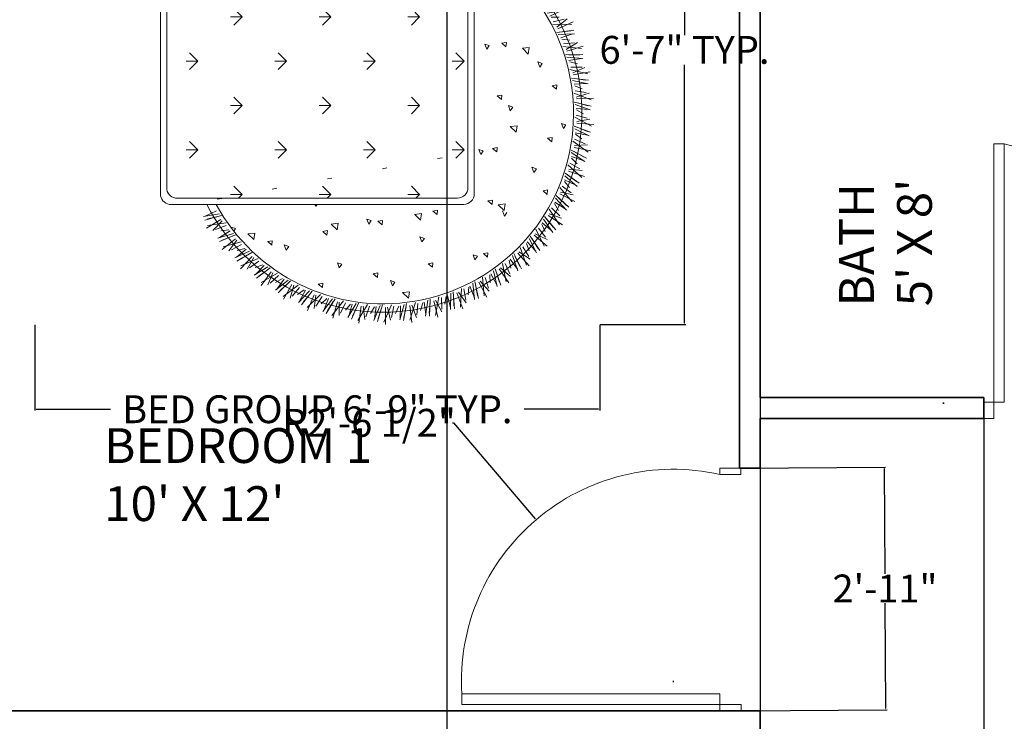
# Model space of a CAD drawing. Units: inches. Extents: x 311 to 754, y 60 to 497.
# Tile 3 of 11: x 388 to 530, y 296 to 396. Entities that reach past the tile are written whole.
import ezdxf

# ---------------------------------------------------------------- set-up
doc = ezdxf.new("R2010")
doc.units = ezdxf.units.IN
doc.header["$MEASUREMENT"] = 0
for name, color, linetype, lineweight in [('A-ANNO-DIMS', 2, 'Continuous', 18), ('A-AREA-IDEN', 1, 'Continuous', 18), ('A-WALL', 7, 'Continuous', 35), ('beds', 70, 'Continuous', 13), ('doors', 210, 'Continuous', 18)]:
    doc.layers.add(name, color=color, linetype=linetype, lineweight=lineweight)
doc.styles.get("Standard").update_dxf_attribs({"font": 'arial.ttf'})
doc.dimstyles.get("Standard").update_dxf_attribs({"dimtxt": 4, "dimasz": 0.18, "dimexe": 0.18, "dimexo": 0.0625, "dimgap": 0.09, "dimtad": 0, "dimtih": 1, "dimtoh": 1, "dimdec": 0, "dimrnd": 6, "dimzin": 0, "dimdsep": 46, "dimlunit": 3, "dimtxsty": 'Standard', "dimcen": 0.09, "dimadec": 0, "dimazin": 0, "dimtfac": 1, "dimtdec": 0, "dimtofl": 0, "dimtmove": 0, "dimatfit": 3, "dimfxl": 1, "dimtolj": 1, "dimtzin": 0, "dimarcsym": 0})

# ---------------------------------------------------------------- blocks, each defined once
blk = doc.blocks.new('A$C57792D97')
for p, q in [((0.6, 2.6235), (0, 2.6235)), ((0, 2.6235), (0, 2.1735)), ((2.1, 2.6235), (0.6, 2.6235)), ((0.6, 2.6235), (0.6, 0.6235)), ((0.6, 0.6235), (0.6, 2.6235)), ((0.6, 2.1735), (0.6, 2.6235)), ((2.1, 0.6235), (2.1, 2.6235)), ((2.7, 2.6235), (2.1, 2.6235)), ((2.1, 2.6235), (2.1, 2.1735)), ((2.7, 2.1735), (2.7, 2.6235)), ((0.6, 2.5735), (0, 2.5735)), ((2.1, 2.5735), (0.6, 2.5735)), ((2.7, 2.5735), (2.1, 2.5735)), ((2.4103, 2.2312), (2.4103, 2.5317)), ((2.2593, 2.3802), (2.5698, 2.3802)), ((0, 2.1735), (0.6, 2.1735)), ((1.5491, 2.1955), (1.5516, 2.1955)), ((2.1, 2.1735), (2.7, 2.1735)), ((0.6, 2.1518), (0.8661, 2.1518)), ((0.6, 1.9518), (1.4767, 1.9518)), ((0.63, 0.6535), (0.63, 1.9518)), ((0.9906, 1.8942), (0.9508, 1.934)), ((1.4149, 1.8942), (1.3751, 1.934)), ((0.9906, 1.8942), (0.9344, 1.8942)), ((0.9906, 1.8942), (0.9508, 1.8544)), ((1.4149, 1.8942), (1.3586, 1.8942)), ((1.4149, 1.8942), (1.3751, 1.8544)), ((2.142, 1.8959), (2.1018, 1.8254)), ((2.1679, 1.8652), (2.1088, 1.8077)), ((2.1584, 1.8544), (2.1201, 1.8188)), ((2.1812, 1.8524), (2.1207, 1.8046)), ((2.1749, 1.8475), (2.1394, 1.7993)), ((2.1799, 1.8155), (2.1465, 1.7971)), ((2.2066, 1.8191), (2.1664, 1.7827)), ((2.249, 1.8154), (2.1711, 1.7709)), ((2.2173, 1.8274), (2.1931, 1.7688)), ((2.2496, 1.8292), (2.2008, 1.7642)), ((2.2713, 1.7954), (2.2055, 1.7458)), ((2.07, 1.7793), (2.07, 0.6535)), ((2.283, 1.7811), (2.2169, 1.7413)), ((2.2607, 1.7859), (2.2181, 1.7554)), ((2.2761, 1.777), (2.2348, 1.7337)), ((2.277, 1.7446), (2.2416, 1.7306)), ((2.304, 1.7449), (2.2596, 1.7138)), ((2.3157, 1.7518), (2.2843, 1.6966)), ((2.3479, 1.7495), (2.2914, 1.6911)), ((0.7785, 1.6821), (0.7387, 1.7219)), ((1.2027, 1.6821), (1.163, 1.7219)), ((1.627, 1.6821), (1.5872, 1.7219)), ((2.0513, 1.6821), (2.0115, 1.7219)), ((2.3456, 1.7359), (2.2627, 1.7015)), ((2.3653, 1.7133), (2.2937, 1.6723)), ((2.3751, 1.6976), (2.3045, 1.6664)), ((2.3535, 1.7051), (2.3075, 1.6802)), ((2.3677, 1.6944), (2.3213, 1.6565)), ((0.7785, 1.6821), (0.7222, 1.6821)), ((0.7785, 1.6821), (0.7387, 1.6423)), ((1.2027, 1.6821), (1.1465, 1.6821)), ((1.2027, 1.6821), (1.163, 1.6423)), ((1.627, 1.6821), (1.5708, 1.6821)), ((1.627, 1.6821), (1.5872, 1.6423)), ((2.0513, 1.6821), (1.995, 1.6821)), ((2.0513, 1.6821), (2.0115, 1.6423)), ((2.3645, 1.6621), (2.3277, 1.6526)), ((2.3913, 1.659), (2.3434, 1.6337)), ((2.4038, 1.6644), (2.3657, 1.6136)), ((2.4355, 1.6581), (2.372, 1.6073)), ((2.4314, 1.6449), (2.3449, 1.6211)), ((2.4482, 1.62), (2.372, 1.5882)), ((2.4559, 1.6032), (2.382, 1.581)), ((2.4354, 1.6134), (2.3867, 1.5944)), ((2.4482, 1.6009), (2.3974, 1.5692)), ((2.2754, 1.598), (2.2534, 1.5939)), ((2.2736, 1.5771), (2.2535, 1.594)), ((2.2736, 1.5771), (2.2754, 1.598)), ((2.441, 1.5693), (2.4032, 1.5645)), ((2.4672, 1.5629), (2.4164, 1.5438)), ((2.4802, 1.5667), (2.4361, 1.5211)), ((2.5109, 1.5564), (2.4416, 1.514)), ((0.9906, 1.47), (0.9508, 1.5097)), ((1.4149, 1.47), (1.3751, 1.5097)), ((1.8391, 1.47), (1.7994, 1.5097)), ((2.3123, 1.541), (2.2911, 1.5481)), ((2.3006, 1.5236), (2.2912, 1.5481)), ((2.3006, 1.5236), (2.3123, 1.541)), ((2.5052, 1.5438), (2.4164, 1.5311)), ((2.5187, 1.517), (2.4392, 1.4951)), ((2.5052, 1.5121), (2.4545, 1.4994)), ((0.9906, 1.47), (0.9344, 1.47)), ((0.9906, 1.47), (0.9508, 1.4302)), ((1.4149, 1.47), (1.3586, 1.47)), ((1.4149, 1.47), (1.3751, 1.4302)), ((1.8391, 1.47), (1.7829, 1.47)), ((1.8391, 1.47), (1.7994, 1.4302)), ((2.5243, 1.4994), (2.4482, 1.4867)), ((2.5163, 1.4981), (2.462, 1.473)), ((2.5052, 1.4677), (2.4672, 1.4677)), ((2.5438, 1.4601), (2.4943, 1.4204)), ((2.5658, 1.4343), (2.4761, 1.4328)), ((2.5304, 1.458), (2.4777, 1.4454)), ((2.573, 1.4461), (2.4989, 1.4127)), ((2.5758, 1.406), (2.4942, 1.3942)), ((2.5791, 1.3878), (2.502, 1.3848)), ((2.5618, 1.4028), (2.5099, 1.3966)), ((2.571, 1.3876), (2.514, 1.3695)), ((2.1596, 1.3147), (2.1502, 1.3392)), ((2.1714, 1.3321), (2.1502, 1.3392)), ((2.1596, 1.3147), (2.1714, 1.3321)), ((2.2534, 1.3469), (2.2315, 1.3429)), ((2.2516, 1.326), (2.2315, 1.3429)), ((2.2516, 1.326), (2.2535, 1.347)), ((2.3632, 1.3229), (2.33, 1.319)), ((2.3584, 1.2918), (2.33, 1.319)), ((2.3584, 1.2918), (2.3632, 1.3229)), ((2.5562, 1.3587), (2.5185, 1.3635)), ((2.6121, 1.3181), (2.523, 1.3279)), ((2.58, 1.346), (2.5261, 1.3402)), ((2.5936, 1.3464), (2.5395, 1.3132)), ((2.6207, 1.3289), (2.5431, 1.305)), ((0.7785, 1.2578), (0.7387, 1.2976)), ((1.2027, 1.2578), (1.163, 1.2976)), ((1.627, 1.2578), (1.5872, 1.2976)), ((2.0513, 1.2578), (2.0115, 1.2976)), ((2.6185, 1.2888), (2.5361, 1.2873)), ((2.6195, 1.2703), (2.5426, 1.277)), ((2.6042, 1.2873), (2.5519, 1.2877)), ((2.6115, 1.2711), (2.5526, 1.2603)), ((0.7785, 1.2578), (0.7222, 1.2578)), ((0.7785, 1.2578), (0.7387, 1.218)), ((1.2027, 1.2578), (1.1465, 1.2578)), ((1.2027, 1.2578), (1.163, 1.218)), ((1.627, 1.2578), (1.5708, 1.2578)), ((1.627, 1.2578), (1.5872, 1.218)), ((2.0513, 1.2578), (1.995, 1.2578)), ((2.0513, 1.2578), (2.0115, 1.218)), ((2.4134, 1.2295), (2.404, 1.254)), ((2.4252, 1.2469), (2.404, 1.254)), ((2.4134, 1.2295), (2.4252, 1.2469)), ((2.5932, 1.2443), (2.5563, 1.2538)), ((2.6152, 1.2287), (2.561, 1.2296)), ((2.6287, 1.2274), (2.5709, 1.2013)), ((2.6435, 1.197), (2.5563, 1.2178)), ((2.6534, 1.2066), (2.5734, 1.1926)), ((2.4947, 1.1445), (2.4728, 1.1404)), ((2.4929, 1.1236), (2.4728, 1.1404)), ((2.4929, 1.1236), (2.4948, 1.1445)), ((2.6462, 1.1671), (2.5642, 1.176)), ((2.6449, 1.1486), (2.5694, 1.1649)), ((2.637, 1.1504), (2.5773, 1.147)), ((2.6319, 1.1675), (2.58, 1.1743)), ((2.6155, 1.1261), (2.5801, 1.1402)), ((0.9906, 1.0457), (0.9508, 1.0855)), ((1.4149, 1.0457), (1.3751, 1.0855)), ((1.8391, 1.0457), (1.7994, 1.0855)), ((2.2315, 1.0959), (2.2095, 1.0919)), ((2.2297, 1.075), (2.2096, 1.0919)), ((2.2297, 1.075), (2.2315, 1.0959)), ((2.6595, 1.0729), (2.5756, 1.1045)), ((2.6353, 1.1079), (2.5817, 1.1156)), ((2.6486, 1.1049), (2.588, 1.0862)), ((0.9906, 1.0457), (0.9344, 1.0457)), ((0.9906, 1.0457), (0.9508, 1.0059)), ((1.4149, 1.0457), (1.3586, 1.0457)), ((1.4149, 1.0457), (1.3751, 1.0059)), ((1.8391, 1.0457), (1.7829, 1.0457)), ((1.8391, 1.0457), (1.7994, 1.0059)), ((2.2725, 1.0206), (2.2631, 1.0451)), ((2.2842, 1.038), (2.2631, 1.0451)), ((2.2725, 1.0206), (2.2843, 1.038)), ((2.6584, 1.0429), (2.5782, 1.062)), ((2.6548, 1.0248), (2.582, 1.0503)), ((2.6705, 1.0812), (2.5894, 1.0774)), ((2.6442, 1.045), (2.5937, 1.0584)), ((2.6598, 0.9477), (2.5805, 0.9897)), ((2.6472, 1.0275), (2.5875, 1.0316)), ((2.6402, 0.9855), (2.588, 0.9999)), ((2.6228, 1.0061), (2.5895, 1.0244)), ((2.3053, 0.9493), (2.272, 0.9455)), ((2.3005, 0.9182), (2.2721, 0.9455)), ((2.3005, 0.9182), (2.3053, 0.9494)), ((2.5263, 0.9355), (2.5169, 0.96)), ((2.538, 0.9528), (2.5169, 0.9599)), ((2.5263, 0.9355), (2.5381, 0.9529)), ((2.655, 0.9181), (2.5778, 0.9471)), ((2.653, 0.9809), (2.5905, 0.97)), ((2.6718, 0.9546), (2.5908, 0.961)), ((2.6412, 0.9221), (2.5927, 0.9416)), ((2.6491, 0.9006), (2.5801, 0.9351)), ((2.6419, 0.9043), (2.5832, 0.9159)), ((2.6151, 0.8861), (2.5843, 0.9085)), ((0.7785, 0.8336), (0.7387, 0.8733)), ((1.2027, 0.8336), (1.163, 0.8733)), ((1.627, 0.8336), (1.5872, 0.8733)), ((2.0513, 0.8336), (2.0115, 0.8733)), ((2.4728, 0.8934), (2.4508, 0.8894)), ((2.471, 0.8725), (2.4509, 0.8894)), ((2.471, 0.8725), (2.4728, 0.8934)), ((2.6444, 0.8236), (2.571, 0.8751)), ((2.6418, 0.8573), (2.5785, 0.8543)), ((2.6297, 0.8635), (2.5797, 0.8843)), ((0.7785, 0.8336), (0.7222, 0.8336)), ((0.7785, 0.8336), (0.7387, 0.7938)), ((1.2027, 0.8336), (1.1465, 0.8336)), ((1.2027, 0.8336), (1.163, 0.7938)), ((1.627, 0.8336), (1.5708, 0.8336)), ((1.627, 0.8336), (1.5872, 0.7938)), ((2.0513, 0.8336), (1.995, 0.8336)), ((2.0513, 0.8336), (2.0115, 0.7938)), ((2.1316, 0.8117), (2.1222, 0.8362)), ((2.1433, 0.8291), (2.1222, 0.8362)), ((2.1316, 0.8117), (2.1434, 0.8291)), ((2.2095, 0.8449), (2.1876, 0.8408)), ((2.2077, 0.824), (2.1876, 0.8408)), ((2.2077, 0.824), (2.2095, 0.8449)), ((2.6359, 0.7948), (2.5629, 0.8332)), ((2.6279, 0.7781), (2.5637, 0.821)), ((2.6212, 0.7827), (2.5644, 0.8015)), ((2.6227, 0.8004), (2.577, 0.8259)), ((2.6572, 0.8289), (2.5776, 0.8454)), ((1.9462, 0.7963), (1.9243, 0.7923)), ((2.6136, 0.7023), (2.5472, 0.7626)), ((2.604, 0.7437), (2.557, 0.7707)), ((2.5923, 0.768), (2.5646, 0.7941)), ((1.683, 0.7477), (1.661, 0.7437)), ((2.3854, 0.7265), (2.376, 0.751)), ((2.3971, 0.7439), (2.376, 0.751)), ((2.3854, 0.7265), (2.3972, 0.7439)), ((2.5915, 0.6593), (2.5332, 0.7099)), ((2.6016, 0.6748), (2.534, 0.7221)), ((2.5892, 0.6821), (2.547, 0.7131)), ((2.6269, 0.706), (2.5501, 0.7323)), ((2.6153, 0.7361), (2.552, 0.7411)), ((0.9906, 0.6214), (0.9508, 0.6612)), ((1.4149, 0.6214), (1.3751, 0.6612)), ((1.4197, 0.6992), (1.3978, 0.6951)), ((1.8391, 0.6214), (1.7994, 0.6612)), ((2.5635, 0.6282), (2.5203, 0.6608)), ((2.5549, 0.6537), (2.5307, 0.6831)), ((2.5855, 0.6646), (2.5315, 0.6905)), ((0.9906, 0.6214), (0.9344, 0.6214)), ((0.9906, 0.6214), (0.9727, 0.6035)), ((1.1564, 0.6506), (1.1345, 0.6466)), ((1.4149, 0.6214), (1.3586, 0.6214)), ((1.4149, 0.6214), (1.397, 0.6035)), ((1.8391, 0.6214), (1.7829, 0.6214)), ((1.8391, 0.6214), (1.8212, 0.6035)), ((2.4508, 0.6424), (2.4289, 0.6383)), ((2.449, 0.6215), (2.4289, 0.6384)), ((2.449, 0.6215), (2.4508, 0.6424)), ((2.5524, 0.5601), (2.4913, 0.6155)), ((2.5815, 0.5878), (2.5085, 0.6236)), ((2.5678, 0.5858), (2.5095, 0.654)), ((2.5737, 0.6192), (2.5116, 0.632)), ((0.6417, 0.5735), (2.05, 0.5735)), ((2.02, 0.6035), (0.6716, 0.6035)), ((0.8932, 0.6021), (0.8712, 0.598)), ((1.3422, 0.5642), (1.3386, 0.5735)), ((1.3422, 0.5642), (1.3485, 0.5735)), ((2.1875, 0.5938), (2.1656, 0.5898)), ((2.1857, 0.5729), (2.1656, 0.5898)), ((2.1857, 0.5729), (2.1876, 0.5938)), ((2.2473, 0.5758), (2.2141, 0.5719)), ((2.2425, 0.5447), (2.2141, 0.572)), ((2.2425, 0.5447), (2.2474, 0.5758)), ((2.5035, 0.545), (2.4831, 0.5772)), ((2.5352, 0.552), (2.4849, 0.5844)), ((2.5405, 0.546), (2.489, 0.6034)), ((2.541, 0.5688), (2.5031, 0.6049)), ((0.8062, 0.5164), (0.8823, 0.5291)), ((0.8118, 0.4988), (0.8913, 0.5207)), ((0.8142, 0.5177), (0.8685, 0.5428)), ((1.8485, 0.5294), (1.8152, 0.5255)), ((1.8437, 0.4983), (1.8153, 0.5256)), ((1.8437, 0.4983), (1.8485, 0.5294)), ((1.9243, 0.5453), (1.9023, 0.5412)), ((1.9225, 0.5244), (1.9024, 0.5412)), ((1.9225, 0.5244), (1.9243, 0.5453)), ((2.2445, 0.5176), (2.2351, 0.5421)), ((2.2445, 0.5176), (2.2562, 0.535)), ((2.5216, 0.4763), (2.4537, 0.5209)), ((2.5178, 0.5084), (2.4578, 0.5289)), ((2.5078, 0.476), (2.4585, 0.551)), ((2.5088, 0.5186), (2.47, 0.5564)), ((0.8196, 0.4594), (0.8889, 0.5018)), ((0.8253, 0.5037), (0.876, 0.5164)), ((0.8253, 0.472), (0.9141, 0.4847)), ((0.8503, 0.4491), (0.8944, 0.4947)), ((0.8633, 0.4529), (0.9141, 0.472)), ((1.4496, 0.483), (1.4163, 0.4791)), ((1.4448, 0.4519), (1.4164, 0.4792)), ((1.4448, 0.4519), (1.4496, 0.483)), ((1.6077, 0.4964), (1.5865, 0.5035)), ((1.596, 0.479), (1.5866, 0.5035)), ((1.596, 0.479), (1.6077, 0.4964)), ((1.661, 0.4967), (1.6391, 0.4927)), ((1.6592, 0.4758), (1.6391, 0.4927)), ((1.6592, 0.4758), (1.661, 0.4967)), ((2.4389, 0.4436), (2.4227, 0.478)), ((2.4712, 0.4466), (2.4253, 0.485)), ((2.4757, 0.4399), (2.4318, 0.5034)), ((2.4893, 0.4525), (2.4356, 0.515)), ((2.4791, 0.4625), (2.446, 0.503)), ((0.8746, 0.4126), (0.9485, 0.4347)), ((0.8823, 0.4149), (0.9331, 0.4466)), ((0.8823, 0.3958), (0.9585, 0.4275)), ((0.8895, 0.4465), (0.9273, 0.4513)), ((0.9592, 0.4578), (0.938, 0.4649)), ((0.9403, 0.459), (0.9381, 0.4649)), ((0.9508, 0.4454), (0.9592, 0.4578)), ((1.0507, 0.4366), (1.0175, 0.4327)), ((1.0459, 0.4055), (1.0175, 0.4328)), ((1.0459, 0.4055), (1.0507, 0.4366)), ((1.3977, 0.4481), (1.3758, 0.4441)), ((1.3959, 0.4272), (1.3758, 0.4441)), ((1.3959, 0.4272), (1.3978, 0.4482)), ((2.4482, 0.3731), (2.3865, 0.4259)), ((2.4485, 0.4055), (2.3915, 0.4334)), ((2.4345, 0.3746), (2.395, 0.4552)), ((2.4409, 0.4167), (2.4071, 0.4591)), ((0.895, 0.3577), (0.9585, 0.4085)), ((0.8951, 0.4024), (0.9438, 0.4214)), ((0.8991, 0.3709), (0.9856, 0.3946)), ((0.9267, 0.3514), (0.9648, 0.4022)), ((0.9392, 0.3568), (0.9872, 0.3821)), ((1.1345, 0.3996), (1.1125, 0.3955)), ((1.1327, 0.3787), (1.1126, 0.3955)), ((1.1327, 0.3787), (1.1345, 0.3996)), ((1.213, 0.3727), (1.1918, 0.3798)), ((1.2013, 0.3553), (1.1919, 0.3798)), ((1.8615, 0.4113), (1.8403, 0.4184)), ((1.8498, 0.3939), (1.8404, 0.4184)), ((1.8498, 0.3939), (1.8615, 0.4113)), ((2.3621, 0.3511), (2.3503, 0.3873)), ((2.3945, 0.35), (2.3538, 0.3939)), ((2.3981, 0.3428), (2.3625, 0.4113)), ((2.4132, 0.3535), (2.3678, 0.4224)), ((2.4043, 0.3648), (2.3766, 0.4092)), ((0.9555, 0.3182), (1.026, 0.3494)), ((0.9628, 0.3214), (1.0092, 0.3592)), ((0.9652, 0.3025), (1.0368, 0.3435)), ((0.966, 0.3537), (1.0029, 0.3631)), ((0.977, 0.3107), (1.023, 0.3356)), ((1.2013, 0.3553), (1.213, 0.3727)), ((2.1153, 0.3261), (2.0941, 0.3332)), ((2.1036, 0.3087), (2.0942, 0.3332)), ((2.1656, 0.3428), (2.1436, 0.3387)), ((2.1638, 0.3219), (2.1437, 0.3388)), ((2.1638, 0.3219), (2.1656, 0.3428)), ((2.3253, 0.265), (2.2888, 0.3389)), ((2.3625, 0.28), (2.3078, 0.3401)), ((2.3668, 0.3121), (2.3138, 0.3469)), ((2.3491, 0.2832), (2.32, 0.3681)), ((2.3607, 0.3242), (2.3324, 0.3704)), ((0.9826, 0.2663), (1.0392, 0.3246)), ((0.9849, 0.2799), (1.0678, 0.3143)), ((1.0148, 0.264), (1.0462, 0.3191)), ((1.0265, 0.2709), (1.0709, 0.302)), ((1.0535, 0.2712), (1.0889, 0.2852)), ((1.4668, 0.2875), (1.4456, 0.2946)), ((1.4551, 0.2701), (1.4457, 0.2946)), ((1.4551, 0.2701), (1.4668, 0.2875)), ((1.9023, 0.2942), (1.8804, 0.2902)), ((1.9005, 0.2733), (1.8804, 0.2902)), ((1.9005, 0.2733), (1.9023, 0.2942)), ((2.1036, 0.3087), (2.1153, 0.3261)), ((2.2529, 0.2032), (2.2346, 0.291)), ((2.2695, 0.2424), (2.2473, 0.2918)), ((2.2743, 0.2689), (2.2671, 0.3063)), ((2.3063, 0.2638), (2.2714, 0.3124)), ((2.309, 0.2562), (2.2823, 0.3286)), ((2.3179, 0.2773), (2.2959, 0.3247)), ((1.0475, 0.2347), (1.1136, 0.2745)), ((1.0544, 0.2388), (1.0957, 0.2821)), ((1.0592, 0.2203), (1.125, 0.27)), ((1.0699, 0.2299), (1.1124, 0.2604)), ((1.0809, 0.1866), (1.1297, 0.2516)), ((1.0815, 0.2004), (1.1594, 0.2449)), ((1.1132, 0.1884), (1.1374, 0.247)), ((1.639, 0.2457), (1.6171, 0.2416)), ((1.6372, 0.2248), (1.6171, 0.2416)), ((1.6372, 0.2248), (1.6391, 0.2457)), ((2.1768, 0.1984), (2.1745, 0.2364)), ((2.208, 0.1893), (2.1795, 0.2419)), ((2.2097, 0.1814), (2.1923, 0.2566)), ((2.227, 0.1881), (2.2001, 0.2661)), ((2.2212, 0.2012), (2.2053, 0.2511)), ((2.2658, 0.1984), (2.2191, 0.2649)), ((2.2741, 0.2296), (2.2258, 0.2708)), ((1.1239, 0.1967), (1.1641, 0.2331)), ((1.1493, 0.1634), (1.2098, 0.2112)), ((1.1507, 0.2003), (1.184, 0.2187)), ((1.1556, 0.1683), (1.1911, 0.2165)), ((1.1626, 0.1506), (1.2217, 0.2081)), ((1.1721, 0.1614), (1.2104, 0.197)), ((1.1885, 0.1199), (1.2287, 0.1904)), ((1.3758, 0.1971), (1.3538, 0.193)), ((1.374, 0.1762), (1.3539, 0.1931)), ((1.374, 0.1762), (1.3758, 0.1971)), ((1.7206, 0.2023), (1.6994, 0.2094)), ((1.7089, 0.1849), (1.6995, 0.2095)), ((1.7089, 0.1849), (1.7206, 0.2024)), ((2.1018, 0.1197), (2.0939, 0.1965)), ((2.1198, 0.1242), (2.1029, 0.2049)), ((2.1157, 0.1379), (2.1062, 0.1893)), ((2.1596, 0.1295), (2.1216, 0.2013)), ((2.1718, 0.1594), (2.129, 0.2063)), ((2.1474, 0.1359), (2.1403, 0.2253)), ((2.1688, 0.1727), (2.1529, 0.2245)), ((1.1873, 0.1336), (1.259, 0.1875)), ((1.2203, 0.1256), (1.237, 0.1868)), ((1.2299, 0.1352), (1.2652, 0.1764)), ((1.2559, 0.1422), (1.2867, 0.1646)), ((1.2592, 0.1054), (1.3133, 0.1604)), ((1.2649, 0.111), (1.2941, 0.1633)), ((1.2741, 0.0944), (1.3255, 0.1588)), ((1.282, 0.1063), (1.3156, 0.1464)), ((1.3007, 0.0806), (1.3651, 0.1431)), ((1.3035, 0.0671), (1.3346, 0.1421)), ((1.7905, 0.1559), (1.7573, 0.152)), ((1.7857, 0.1248), (1.7573, 0.152)), ((1.7857, 0.1248), (1.7906, 0.1559)), ((1.9871, 0.072), (1.9889, 0.1491)), ((2.0054, 0.0742), (1.9988, 0.1564)), ((2.0456, 0.0745), (2.0169, 0.1505)), ((2.0614, 0.1027), (2.0249, 0.1545)), ((2.0343, 0.0824), (2.0385, 0.172)), ((2.0601, 0.1162), (2.0509, 0.1696)), ((2.0714, 0.1407), (2.0737, 0.1787)), ((2.1011, 0.1277), (2.0794, 0.1835)), ((1.3344, 0.0768), (1.3433, 0.1396)), ((1.3427, 0.0876), (1.3725, 0.1328)), ((1.3677, 0.0977), (1.3954, 0.1238)), ((1.3755, 0.0616), (1.4223, 0.1229)), ((1.3804, 0.0679), (1.4028, 0.1234)), ((1.3916, 0.0525), (1.4346, 0.1229)), ((1.3981, 0.0653), (1.4264, 0.1093)), ((1.4198, 0.0422), (1.4758, 0.1123)), ((1.4243, 0.0292), (1.4458, 0.1075)), ((1.4537, 0.0427), (1.4546, 0.1061)), ((1.4606, 0.0544), (1.4845, 0.103)), ((1.4841, 0.0676), (1.5083, 0.0969)), ((1.4964, 0.0327), (1.5351, 0.0995)), ((1.5005, 0.0397), (1.5158, 0.0975)), ((1.5135, 0.0258), (1.5473, 0.101)), ((1.5428, 0.0191), (1.5896, 0.0956)), ((1.7442, 0.0214), (1.7651, 0.0956)), ((1.7625, 0.0189), (1.7765, 0.1002)), ((1.7925, 0.0197), (1.8188, 0.1054)), ((1.8259, 0.046), (1.8303, 0.1)), ((1.8429, 0.0669), (1.8547, 0.1031)), ((1.8685, 0.047), (1.8614, 0.1064)), ((1.8672, 0.039), (1.8787, 0.1154)), ((1.8852, 0.0532), (1.8888, 0.1054)), ((1.8857, 0.0389), (1.8894, 0.1213)), ((1.9256, 0.0342), (1.9067, 0.1132)), ((1.9448, 0.0601), (1.9151, 0.1162)), ((1.9154, 0.0434), (1.9307, 0.1318)), ((1.9452, 0.0737), (1.9428, 0.1279)), ((1.9595, 0.0966), (1.9666, 0.134)), ((1.9873, 0.08), (1.9728, 0.1381)), ((2.0031, 0.0883), (2.0001, 0.1405)), ((1.5183, 0.0393), (1.5409, 0.0865)), ((1.5489, 0.0067), (1.5603, 0.0871)), ((1.5763, 0.0238), (1.5693, 0.0868)), ((1.5817, 0.0362), (1.5994, 0.0875)), ((1.6034, 0.0523), (1.6237, 0.0845)), ((1.6199, 0.0192), (1.65, 0.0903)), ((1.6232, 0.0266), (1.631, 0.086)), ((1.6378, 0.0145), (1.6619, 0.0934)), ((1.6409, 0.0285), (1.6573, 0.0782)), ((1.6677, 0.0115), (1.7045, 0.0933)), ((1.6753, 0), (1.6766, 0.0812)), ((1.7004, 0.0204), (1.6855, 0.0821)), ((1.7041, 0.0334), (1.7152, 0.0865)), ((1.7236, 0.0521), (1.7398, 0.0865)), ((1.7465, 0.0291), (1.7469, 0.0889)), ((1.7638, 0.0332), (1.7739, 0.0845)), ((1.8015, 0.0092), (1.7926, 0.09)), ((1.8238, 0.0326), (1.8014, 0.0919))]:
    blk.add_line(p, q)
at = {"linetype": 'ByBlock'}
for p, q in [((0.3217, 2.5511), (0.3189, 2.5483)), ((0.3189, 2.5483), (0.3189, 2.3511)), ((0.5475, 2.5511), (0.3217, 2.5511)), ((0.3375, 2.5469), (0.3303, 2.5397)), ((0.3346, 2.5426), (0.3332, 2.5369)), ((0.3403, 2.5454), (0.3346, 2.5426)), ((0.3803, 2.5469), (0.3375, 2.5469)), ((0.3746, 2.5454), (0.3403, 2.5454)), ((0.3475, 2.5269), (0.3403, 2.5454)), ((0.3675, 2.5269), (0.3746, 2.5454)), ((0.3746, 2.5454), (0.3803, 2.5426)), ((0.386, 2.5397), (0.3803, 2.5469)), ((0.3803, 2.5426), (0.3818, 2.5369)), ((0.5475, 2.5511), (0.5503, 2.5483)), ((0.5503, 2.5483), (0.5503, 2.3511)), ((0.3303, 2.5397), (0.3303, 2.3683)), ((0.3332, 2.5369), (0.3332, 2.4983)), ((0.3332, 2.5369), (0.346, 2.524)), ((0.3332, 2.4983), (0.336, 2.4911)), ((0.346, 2.524), (0.3475, 2.5269)), ((0.346, 2.4597), (0.346, 2.524)), ((0.3475, 2.5269), (0.3675, 2.5269)), ((0.3689, 2.524), (0.3675, 2.5269)), ((0.3818, 2.5369), (0.3689, 2.524)), ((0.3689, 2.4597), (0.3689, 2.524)), ((0.3818, 2.4983), (0.3789, 2.4911)), ((0.3818, 2.5369), (0.3818, 2.4983)), ((0.386, 2.3668), (0.386, 2.5397)), ((0.3989, 2.4597), (0.3989, 2.5354)), ((0.3989, 2.5354), (0.5418, 2.5354)), ((0.5418, 2.5354), (0.5418, 2.4597)), ((0.336, 2.4911), (0.3403, 2.484)), ((0.3403, 2.484), (0.3417, 2.474)), ((0.3417, 2.474), (0.3417, 2.4597)), ((0.3417, 2.4326), (0.3417, 2.4597)), ((0.346, 2.4597), (0.346, 2.3826)), ((0.3689, 2.4597), (0.3689, 2.3826)), ((0.3746, 2.484), (0.3732, 2.474)), ((0.3732, 2.474), (0.3732, 2.4597)), ((0.3732, 2.4326), (0.3732, 2.4597)), ((0.3789, 2.4911), (0.3746, 2.484)), ((0.5418, 2.4597), (0.3989, 2.4597)), ((0.3989, 2.4426), (0.3989, 2.4568)), ((0.3989, 2.4568), (0.5361, 2.4568)), ((0.4675, 2.4568), (0.4675, 2.4426)), ((0.4789, 2.4568), (0.4789, 2.4426)), ((0.4903, 2.4568), (0.4903, 2.4426)), ((0.5018, 2.4568), (0.5018, 2.4426)), ((0.5132, 2.4568), (0.5132, 2.4426)), ((0.5246, 2.4568), (0.5246, 2.4426)), ((0.5361, 2.4568), (0.5361, 2.4426)), ((0.3332, 2.4083), (0.336, 2.4154)), ((0.3332, 2.3697), (0.3332, 2.4083)), ((0.336, 2.4154), (0.3403, 2.4226)), ((0.3403, 2.4226), (0.3417, 2.4326)), ((0.3746, 2.4226), (0.3732, 2.4326)), ((0.3789, 2.4154), (0.3746, 2.4226)), ((0.3818, 2.4083), (0.3789, 2.4154)), ((0.3818, 2.3697), (0.3818, 2.4083)), ((0.5361, 2.4426), (0.3989, 2.4426)), ((0.3989, 2.4197), (0.3989, 2.4111)), ((0.4103, 2.4197), (0.3989, 2.4197)), ((0.3989, 2.4111), (0.4103, 2.4111)), ((0.3989, 2.404), (0.3989, 2.3954)), ((0.4103, 2.404), (0.3989, 2.404)), ((0.4103, 2.4111), (0.4103, 2.4197)), ((0.4103, 2.3954), (0.4103, 2.404)), ((0.4275, 2.4197), (0.416, 2.4197)), ((0.416, 2.4197), (0.416, 2.4111)), ((0.416, 2.4111), (0.4275, 2.4111)), ((0.416, 2.404), (0.416, 2.3954)), ((0.4275, 2.404), (0.416, 2.404)), ((0.4275, 2.4111), (0.4275, 2.4197)), ((0.4275, 2.3954), (0.4275, 2.404)), ((0.4332, 2.4197), (0.4332, 2.4111)), ((0.4446, 2.4197), (0.4332, 2.4197)), ((0.4332, 2.4111), (0.4446, 2.4111)), ((0.4332, 2.404), (0.4332, 2.3954)), ((0.4446, 2.404), (0.4332, 2.404)), ((0.4446, 2.4111), (0.4446, 2.4197)), ((0.4446, 2.3954), (0.4446, 2.404)), ((0.4575, 2.4011), (0.4575, 2.4268)), ((0.4575, 2.4268), (0.5418, 2.4268)), ((0.5418, 2.4011), (0.4575, 2.4011)), ((0.4718, 2.424), (0.4761, 2.424)), ((0.4718, 2.4197), (0.4718, 2.424)), ((0.4761, 2.4197), (0.4718, 2.4197)), ((0.4718, 2.4083), (0.4761, 2.4083)), ((0.4718, 2.404), (0.4718, 2.4083)), ((0.4761, 2.404), (0.4718, 2.404)), ((0.4761, 2.424), (0.4761, 2.4197)), ((0.4761, 2.4083), (0.4761, 2.404)), ((0.4975, 2.424), (0.5018, 2.424)), ((0.4975, 2.4197), (0.4975, 2.424)), ((0.5018, 2.4197), (0.4975, 2.4197)), ((0.4975, 2.4083), (0.5018, 2.4083)), ((0.4975, 2.404), (0.4975, 2.4083)), ((0.5018, 2.404), (0.4975, 2.404)), ((0.5018, 2.424), (0.5018, 2.4197)), ((0.5018, 2.4083), (0.5018, 2.404)), ((0.5232, 2.4197), (0.5232, 2.424)), ((0.5232, 2.424), (0.5275, 2.424)), ((0.5275, 2.4197), (0.5232, 2.4197)), ((0.5232, 2.4083), (0.5275, 2.4083)), ((0.5232, 2.404), (0.5232, 2.4083)), ((0.5275, 2.404), (0.5232, 2.404)), ((0.5275, 2.424), (0.5275, 2.4197)), ((0.5275, 2.4083), (0.5275, 2.404)), ((0.5418, 2.4268), (0.5418, 2.4011)), ((0.2789, 2.3502), (0.2854, 2.3565)), ((0.2854, 2.3565), (0.2932, 2.3525)), ((0.2902, 2.3608), (0.294, 2.3648)), ((0.2932, 2.3525), (0.2902, 2.3608)), ((0.3053, 2.3601), (0.2937, 2.3497)), ((0.294, 2.3648), (0.2975, 2.3621)), ((0.2955, 2.3663), (0.298, 2.3689)), ((0.2975, 2.3621), (0.2955, 2.3663)), ((0.298, 2.3689), (0.3033, 2.3669)), ((0.3053, 2.3628), (0.3023, 2.3631)), ((0.3023, 2.3631), (0.3053, 2.3601)), ((0.3033, 2.3669), (0.3063, 2.3696)), ((0.3068, 2.3648), (0.3053, 2.3628)), ((0.3063, 2.3696), (0.3103, 2.3737)), ((0.3126, 2.3694), (0.3068, 2.3648)), ((0.3103, 2.3737), (0.3189, 2.3768)), ((0.3189, 2.3711), (0.3126, 2.3694)), ((0.3303, 2.3683), (0.3375, 2.3597)), ((0.3332, 2.3697), (0.346, 2.3826)), ((0.3346, 2.364), (0.3332, 2.3697)), ((0.3403, 2.3611), (0.3346, 2.364)), ((0.3375, 2.3597), (0.3542, 2.3597)), ((0.3475, 2.3797), (0.3403, 2.3611)), ((0.3543, 2.3611), (0.3403, 2.3611)), ((0.346, 2.3826), (0.3475, 2.3797)), ((0.3475, 2.3797), (0.3675, 2.3797)), ((0.3518, 2.3447), (0.3538, 2.354)), ((0.3538, 2.354), (0.3546, 2.3654)), ((0.3546, 2.3654), (0.3589, 2.3654)), ((0.3589, 2.3654), (0.3587, 2.3531)), ((0.3746, 2.3611), (0.3588, 2.3611)), ((0.3588, 2.3597), (0.3789, 2.3597)), ((0.3689, 2.3826), (0.3675, 2.3797)), ((0.3675, 2.3797), (0.3746, 2.3611)), ((0.3818, 2.3697), (0.3689, 2.3826)), ((0.3746, 2.3611), (0.3803, 2.364)), ((0.3789, 2.3597), (0.386, 2.3668)), ((0.3803, 2.364), (0.3818, 2.3697)), ((0.3989, 2.3954), (0.4103, 2.3954)), ((0.4103, 2.3883), (0.3989, 2.3883)), ((0.3989, 2.3883), (0.3989, 2.3797)), ((0.3989, 2.3797), (0.4103, 2.3797)), ((0.4103, 2.3711), (0.3989, 2.3711)), ((0.3989, 2.3711), (0.3989, 2.3626)), ((0.3989, 2.3626), (0.4103, 2.3626)), ((0.4103, 2.3797), (0.4103, 2.3883)), ((0.4103, 2.3626), (0.4103, 2.3711)), ((0.416, 2.3954), (0.4275, 2.3954)), ((0.4275, 2.3868), (0.416, 2.3868)), ((0.416, 2.3868), (0.416, 2.3783)), ((0.416, 2.3783), (0.4275, 2.3783)), ((0.416, 2.3711), (0.416, 2.3626)), ((0.4275, 2.3711), (0.416, 2.3711)), ((0.416, 2.3626), (0.4275, 2.3626)), ((0.4275, 2.3783), (0.4275, 2.3868)), ((0.4275, 2.3626), (0.4275, 2.3711)), ((0.4332, 2.3954), (0.4446, 2.3954)), ((0.4446, 2.3868), (0.4332, 2.3868)), ((0.4332, 2.3868), (0.4332, 2.3783)), ((0.4332, 2.3783), (0.4446, 2.3783)), ((0.4332, 2.3711), (0.4332, 2.3626)), ((0.4446, 2.3711), (0.4332, 2.3711)), ((0.4332, 2.3626), (0.4446, 2.3626)), ((0.4446, 2.3783), (0.4446, 2.3868)), ((0.4446, 2.3626), (0.4446, 2.3711)), ((0.4661, 2.394), (0.4803, 2.394)), ((0.4661, 2.3883), (0.4661, 2.394)), ((0.4803, 2.3883), (0.4661, 2.3883)), ((0.4661, 2.3726), (0.4661, 2.364)), ((0.4803, 2.3726), (0.4661, 2.3726)), ((0.4661, 2.364), (0.4803, 2.364)), ((0.4803, 2.394), (0.4803, 2.3883)), ((0.4803, 2.364), (0.4803, 2.3726)), ((0.4861, 2.3883), (0.4861, 2.394)), ((0.4861, 2.394), (0.5003, 2.394)), ((0.5003, 2.3883), (0.4861, 2.3883)), ((0.5003, 2.3726), (0.4861, 2.3726)), ((0.4861, 2.3726), (0.4861, 2.364)), ((0.4861, 2.364), (0.5003, 2.364)), ((0.5003, 2.394), (0.5003, 2.3883)), ((0.5003, 2.364), (0.5003, 2.3726)), ((0.5061, 2.3883), (0.5061, 2.394)), ((0.5061, 2.394), (0.5203, 2.394)), ((0.5203, 2.3883), (0.5061, 2.3883)), ((0.5203, 2.3726), (0.5061, 2.3726)), ((0.5061, 2.3726), (0.5061, 2.364)), ((0.5061, 2.364), (0.5203, 2.364)), ((0.5203, 2.394), (0.5203, 2.3883)), ((0.5203, 2.364), (0.5203, 2.3726)), ((0.5261, 2.3883), (0.5261, 2.394)), ((0.5261, 2.394), (0.5403, 2.394)), ((0.5403, 2.3883), (0.5261, 2.3883)), ((0.5403, 2.3726), (0.5261, 2.3726)), ((0.5261, 2.3726), (0.5261, 2.364)), ((0.5261, 2.364), (0.5403, 2.364)), ((0.5403, 2.394), (0.5403, 2.3883)), ((0.5403, 2.364), (0.5403, 2.3726)), ((0.2532, 2.3027), (0.2546, 2.31)), ((0.2546, 2.31), (0.2624, 2.31)), ((0.2563, 2.3158), (0.2584, 2.3224)), ((0.2624, 2.31), (0.2563, 2.3158)), ((0.2584, 2.3224), (0.2676, 2.3221)), ((0.2592, 2.3253), (0.2618, 2.334)), ((0.2676, 2.3221), (0.2592, 2.3253)), ((0.2618, 2.334), (0.2705, 2.3331)), ((0.2746, 2.3331), (0.265, 2.3059)), ((0.2683, 2.3394), (0.2738, 2.3452)), ((0.2706, 2.3331), (0.2683, 2.3394)), ((0.2738, 2.3452), (0.2804, 2.3412)), ((0.2937, 2.3497), (0.2748, 2.3336)), ((0.2804, 2.3412), (0.2789, 2.3502)), ((0.3189, 2.3511), (0.3217, 2.3483)), ((0.3217, 2.3483), (0.3525, 2.3483)), ((0.3425, 2.3129), (0.3477, 2.3166)), ((0.3437, 2.3062), (0.3425, 2.3129)), ((0.3474, 2.3242), (0.3483, 2.3311)), ((0.3477, 2.3166), (0.3474, 2.3242)), ((0.3483, 2.3311), (0.3518, 2.3447)), ((0.352, 2.3175), (0.3512, 2.3158)), ((0.3512, 2.3158), (0.3544, 2.3126)), ((0.3552, 2.3386), (0.3518, 2.325)), ((0.3518, 2.325), (0.352, 2.3175)), ((0.3544, 2.3126), (0.3549, 2.3056)), ((0.3587, 2.3531), (0.3552, 2.3386)), ((0.3575, 2.3483), (0.5475, 2.3483)), ((0.5503, 2.3511), (0.5475, 2.3483)), ((0.2621, 2.3001), (0.2532, 2.3027)), ((0.2546, 2.2958), (0.2621, 2.3001)), ((0.2558, 2.29), (0.2546, 2.2958)), ((0.2647, 2.2903), (0.2558, 2.29)), ((0.2578, 2.2825), (0.2647, 2.2903)), ((0.2601, 2.2767), (0.2578, 2.2825)), ((0.2685, 2.2793), (0.2601, 2.2767)), ((0.2644, 2.2715), (0.2685, 2.2793)), ((0.2682, 2.268), (0.2644, 2.2715)), ((0.265, 2.3059), (0.2691, 2.2842)), ((0.2763, 2.2715), (0.2682, 2.268)), ((0.2691, 2.2842), (0.2818, 2.2718)), ((0.2728, 2.2637), (0.2763, 2.2715)), ((0.2774, 2.2596), (0.2728, 2.2637)), ((0.2835, 2.2672), (0.2774, 2.2596)), ((0.2818, 2.2718), (0.2986, 2.2646)), ((0.2827, 2.2585), (0.2835, 2.2672)), ((0.2939, 2.262), (0.2873, 2.2562)), ((0.2942, 2.2541), (0.2939, 2.262)), ((0.2986, 2.2646), (0.3159, 2.266)), ((0.3029, 2.262), (0.2997, 2.2527)), ((0.3049, 2.2536), (0.3029, 2.262)), ((0.3133, 2.262), (0.3098, 2.2541)), ((0.3171, 2.2541), (0.3133, 2.262)), ((0.3159, 2.266), (0.3312, 2.2741)), ((0.3292, 2.2596), (0.3223, 2.2654)), ((0.3223, 2.2654), (0.3231, 2.2559)), ((0.3347, 2.2631), (0.3292, 2.2596)), ((0.3312, 2.2741), (0.3422, 2.288)), ((0.3402, 2.266), (0.3335, 2.2709)), ((0.3335, 2.2709), (0.3347, 2.2631)), ((0.3445, 2.2712), (0.3402, 2.266)), ((0.3492, 2.2776), (0.3405, 2.2793)), ((0.3405, 2.2793), (0.3445, 2.2712)), ((0.3422, 2.288), (0.3437, 2.3062)), ((0.3541, 2.2915), (0.3448, 2.2906)), ((0.3448, 2.2906), (0.3529, 2.2842)), ((0.3549, 2.3056), (0.3466, 2.3042)), ((0.3466, 2.3042), (0.3546, 2.2993)), ((0.3529, 2.2842), (0.3492, 2.2776)), ((0.3546, 2.2993), (0.3541, 2.2915)), ((0.2873, 2.2562), (0.2827, 2.2585)), ((0.2997, 2.2527), (0.2942, 2.2541)), ((0.3098, 2.2541), (0.3049, 2.2536)), ((0.3231, 2.2559), (0.3171, 2.2541))]:
    blk.add_line(p, q, dxfattribs=at)
for centre, radius in [((2.4068, 2.3792), 0.1082), ((2.4128, 2.3792), 0.062)]:
    blk.add_circle(centre, radius)
for centre, radius, start, end in [((0.8117, 1.4495), 1.1155, 75.3755, 98.4519), ((0.7133, 2.123), 0.4349, 62.6153, 98.6623), ((0.9995, 2.5566), 0.3518, 180.6066, 203.849), ((1.2711, 1.6927), 0.8548, 85.0132, 101.9962), ((-2.6554, 2.4937), 4.0011, 355.9906, 0.7251), ((1.5803, 0.4369), 2.1259, 84.0997, 95.547), ((7.229, 2.8402), 5.8612, 182.80995, 184.16642), ((1.505, 1.754), 0.7941, 71.9705, 99.0452), ((2.0384, 6.4739), 3.9297, 266.5056, 270.1818), ((2.5231, 2.3654), 0.505, 159.2551, 197.4606), ((0.9942, 1.5092), 1.0245, 76.8495, 84.445), ((1.6997, 1.5092), 1.0245, 76.8495, 84.445), ((6.5168, 1.1676), 5.2262, 165.6998, 168.4122), ((1.7461, 2.3905), 1.0686, 178.7205, 189.3246), ((2.4516, 2.3905), 1.0686, 178.7205, 189.3246), ((1.0382, 2.187), 0.3479, 146.8128, 174.9884), ((1.3553, 2.3447), 0.1322, 217.4973, 261.5591), ((2.6076, 3.8927), 1.7717, 246.8027, 251.3608), ((0.9964, 4.7934), 2.5939, 263.2521, 270.4789), ((1.1218, 3.4256), 1.2305, 265.1643, 280.0187), ((1.5587, 3.1365), 0.9332, 260.0314, 280.1788), ((1.8907, 2.8521), 0.6558, 255.2386, 283.2855), ((1.0153, 0.392), 1.7661, 72.4208, 94.846), ((0.7898, 0.8867), 1.2674, 53.0057, 86.5496), ((2.0108, 3.233), 1.2462, 248.2311, 274.1028), ((1.991, 2.6169), 0.8413, 238.5747, 277.4412), ((1.6653, 1.0079), 0.9493, 207.2312, 62.7432), ((1.6653, 1.0079), 0.9093, 208.5361, 61.4369), ((0.6518, 0.6244), 0.0518, 180.9151, 258.7324), ((0.6787, 0.6517), 0.0487, 177.8916, 261.664), ((2.02, 0.6535), 0.05, 270, 0), ((2.05, 0.6235), 0.05, 270, 0)]:
    blk.add_arc(centre, radius, start, end)
blk = doc.blocks.new('*D110')
at = {"layer": 'A-ANNO-DIMS', "color": 0, "lineweight": -2, "transparency": 16777216}
for p, q in [((390.57, 352.66), (390.57, 340.37)), ((471.73, 352.66), (471.73, 340.37)), ((390.75, 340.55), (401.41, 340.55)), ((471.55, 340.55), (460.89, 340.55))]:
    blk.add_line(p, q, dxfattribs=at)
at = {"layer": 'A-ANNO-DIMS', "color": 0, "transparency": 16777216}
for points in [[(390.75, 340.58), (390.75, 340.52), (390.57, 340.55)], [(471.55, 340.58), (471.55, 340.52), (471.73, 340.55)]]:
    blk.add_solid(points, dxfattribs=at)
at = {"layer": 'Defpoints', "color": 0, "transparency": 16777216}
for p in [(390.57, 352.73), (471.73, 352.73), (471.73, 340.55)]:
    blk.add_point(p, dxfattribs=at)
at = {"layer": 'A-ANNO-DIMS', "color": 0, "transparency": 16777216, "insert": (431.15, 340.55), "char_height": 4, "attachment_point": 5}
blk.add_mtext('\\A1;BED GROUP 6\'-9" TYP.', dxfattribs=at)
blk = doc.blocks.new('*D111')
at = {"layer": 'A-ANNO-DIMS', "color": 0, "lineweight": -2, "transparency": 16777216}
for p, q in [((471.79, 431.59), (484.09, 431.59)), ((483.91, 431.41), (483.91, 394.29)), ((483.91, 352.91), (483.91, 390.03)), ((471.79, 352.73), (484.09, 352.73))]:
    blk.add_line(p, q, dxfattribs=at)
at = {"layer": 'A-ANNO-DIMS', "color": 0, "transparency": 16777216}
for points in [[(483.88, 431.41), (483.94, 431.41), (483.91, 431.59)], [(483.88, 352.91), (483.94, 352.91), (483.91, 352.73)]]:
    blk.add_solid(points, dxfattribs=at)
at = {"layer": 'Defpoints', "color": 0, "transparency": 16777216}
for p in [(471.73, 431.59), (483.91, 431.59), (471.73, 352.73)]:
    blk.add_point(p, dxfattribs=at)
at = {"layer": 'A-ANNO-DIMS', "color": 0, "transparency": 16777216, "insert": (483.91, 392.16), "char_height": 4, "attachment_point": 5}
blk.add_mtext('\\A1;6\'-7" TYP.', dxfattribs=at)
blk = doc.blocks.new('*D129')
at = {"layer": 'A-ANNO-DIMS', "color": 0, "lineweight": -2, "transparency": 16777216}
for p, q in [((491.87, 332.1), (512.78, 332.24)), ((512.61, 332.06), (512.71, 316.9)), ((512.84, 297.56), (512.73, 312.71)), ((492.1, 297.24), (513.02, 297.38))]:
    blk.add_line(p, q, dxfattribs=at)
at = {"layer": 'A-ANNO-DIMS', "color": 0, "transparency": 16777216}
for points in [[(512.64, 332.06), (512.58, 332.06), (512.6, 332.24)], [(512.87, 297.56), (512.81, 297.56), (512.84, 297.38)]]:
    blk.add_solid(points, dxfattribs=at)
at = {"layer": 'Defpoints', "color": 0, "transparency": 16777216}
for p in [(491.8, 332.1), (492.04, 297.24), (512.84, 297.38)]:
    blk.add_point(p, dxfattribs=at)
at = {"layer": 'A-ANNO-DIMS', "color": 0, "transparency": 16777216, "insert": (512.72, 314.81), "char_height": 4, "attachment_point": 5}
blk.add_mtext('\\A1;2\'-11"', dxfattribs=at)
blk = doc.blocks.new('*D132')
at = {"layer": 'A-ANNO-DIMS', "color": 0, "lineweight": -2, "transparency": 16777216}
for p, q in [((526.91, 339.18), (526.91, 66.26)), ((560.82, 339.18), (560.82, 66.26)), ((527.09, 66.44), (536.87, 66.44)), ((560.64, 66.44), (550.86, 66.44))]:
    blk.add_line(p, q, dxfattribs=at)
at = {"layer": 'A-ANNO-DIMS', "color": 0, "transparency": 16777216}
for points in [[(527.09, 66.47), (527.09, 66.41), (526.91, 66.44)], [(560.64, 66.47), (560.64, 66.41), (560.82, 66.44)]]:
    blk.add_solid(points, dxfattribs=at)
at = {"layer": 'Defpoints', "color": 0, "transparency": 16777216}
for p in [(526.91, 339.24), (560.82, 339.24), (526.91, 66.44)]:
    blk.add_point(p, dxfattribs=at)
at = {"layer": 'A-ANNO-DIMS', "color": 0, "transparency": 16777216, "insert": (543.87, 66.44), "char_height": 4, "attachment_point": 5}
blk.add_mtext('\\A1;2\'-10"', dxfattribs=at)
blk = doc.blocks.new('*D134')
at = {"layer": 'A-ANNO-DIMS', "color": 0, "lineweight": -2, "transparency": 16777216}
for p, q in [((494.8, 342.18), (494.8, 66.26)), ((563.8, 342.18), (563.8, 66.26)), ((494.98, 66.44), (523.9, 66.44)), ((563.62, 66.44), (534.71, 66.44))]:
    blk.add_line(p, q, dxfattribs=at)
at = {"layer": 'A-ANNO-DIMS', "color": 0, "transparency": 16777216}
for points in [[(494.98, 66.47), (494.98, 66.41), (494.8, 66.44)], [(563.62, 66.47), (563.62, 66.41), (563.8, 66.44)]]:
    blk.add_solid(points, dxfattribs=at)
at = {"layer": 'Defpoints', "color": 0, "transparency": 16777216}
for p in [(494.8, 342.24), (563.8, 342.24), (563.8, 66.44)]:
    blk.add_point(p, dxfattribs=at)
at = {"layer": 'A-ANNO-DIMS', "color": 0, "transparency": 16777216, "insert": (529.3, 66.44), "char_height": 4, "attachment_point": 5}
blk.add_mtext('\\A1;5\'-9"', dxfattribs=at)
blk = doc.blocks.new('*D136')
at = {"layer": 'A-ANNO-DIMS', "color": 0, "lineweight": -2, "transparency": 16777216}
for p, q in [((371.8, 294.3), (371.8, 486.86)), ((449.8, 294.3), (449.8, 486.86)), ((371.98, 486.68), (405.39, 486.68)), ((449.62, 486.68), (416.22, 486.68))]:
    blk.add_line(p, q, dxfattribs=at)
at = {"layer": 'A-ANNO-DIMS', "color": 0, "transparency": 16777216}
for points in [[(371.98, 486.71), (371.98, 486.65), (371.8, 486.68)], [(449.62, 486.71), (449.62, 486.65), (449.8, 486.68)]]:
    blk.add_solid(points, dxfattribs=at)
at = {"layer": 'Defpoints', "color": 0, "transparency": 16777216}
for p in [(371.8, 486.68), (371.8, 294.24), (449.8, 294.24)]:
    blk.add_point(p, dxfattribs=at)
at = {"layer": 'A-ANNO-DIMS', "color": 0, "transparency": 16777216, "insert": (410.8, 486.68), "char_height": 4, "attachment_point": 5}
blk.add_mtext('\\A1;6\'-6"', dxfattribs=at)
blk = doc.blocks.new('*D153')
at = {"layer": 'A-ANNO-DIMS', "color": 0, "lineweight": -2, "transparency": 16777216}
for p, q in [((450.56, 338.6), (450.74, 338.6)), ((450.74, 338.6), (462.46, 324.81)), ((482.22, 301.47), (482.4, 301.47)), ((482.31, 301.38), (482.31, 301.56))]:
    blk.add_line(p, q, dxfattribs=at)
at = {"layer": 'A-ANNO-DIMS', "color": 0, "transparency": 16777216}
blk.add_solid([(462.48, 324.83), (462.44, 324.79), (462.58, 324.68)], dxfattribs=at)
at = {"layer": 'Defpoints', "color": 0, "transparency": 16777216}
for p in [(462.58, 324.68), (482.31, 301.47)]:
    blk.add_point(p, dxfattribs=at)
at = {"layer": 'A-ANNO-DIMS', "color": 0, "transparency": 16777216, "insert": (438.58, 338.6), "char_height": 4, "attachment_point": 5}
blk.add_mtext('\\A1;R2\'-6 1/2"', dxfattribs=at)
blk = doc.blocks.new('*D155')
at = {"layer": 'A-ANNO-DIMS', "color": 0, "lineweight": -2, "transparency": 16777216}
for p, q in [((569.03, 379.51), (551.21, 365.35)), ((569.21, 379.51), (569.03, 379.51)), ((521.05, 341.43), (521.23, 341.43)), ((521.14, 341.34), (521.14, 341.52))]:
    blk.add_line(p, q, dxfattribs=at)
at = {"layer": 'A-ANNO-DIMS', "color": 0, "transparency": 16777216}
blk.add_solid([(551.19, 365.37), (551.23, 365.32), (551.07, 365.23)], dxfattribs=at)
at = {"layer": 'Defpoints', "color": 0, "transparency": 16777216}
for p in [(551.07, 365.23), (521.14, 341.43)]:
    blk.add_point(p, dxfattribs=at)
at = {"layer": 'A-ANNO-DIMS', "color": 0, "transparency": 16777216, "insert": (576.53, 379.51), "char_height": 4, "attachment_point": 5}
blk.add_mtext('\\A1;R3\'-2"', dxfattribs=at)

msp = doc.modelspace()

# ---------------------------------------------------------------- linework, layer by layer
at = {"layer": 'A-WALL'}
for p, q in [((491.8, 438.24), (491.8, 332.1)), ((494.8, 438.24), (494.8, 342.24)), ((526.91, 342.24), (494.8, 342.24)), ((526.91, 339.24), (526.91, 342.24)), ((526.91, 342.24), (526.91, 342.24)), ((494.8, 339.24), (494.8, 332.1)), ((526.91, 339.24), (494.8, 339.24)), ((491.8, 332.1), (494.8, 332.1)), ((494.8, 297.24), (371.8, 297.24)), ((494.8, 297.24), (494.8, 294.24))]:
    msp.add_line(p, q, dxfattribs=at)
at = {"layer": 'doors'}
for points in [[(528.34, 341.55), (529.86, 341.55), (529.86, 378.66), (528.34, 378.66)], [(526.91, 339.24), (528.35, 339.24), (528.35, 341.55), (526.91, 341.55)], [(526.91, 339.24), (526.91, 339.24), (526.91, 341.22), (526.91, 341.22)], [(492.01, 331.19), (488.98, 331.19), (488.98, 332.1), (492.01, 332.1)], [(451.9, 299.67), (451.9, 298.15), (489.01, 298.15), (489.01, 299.67)], [(492.04, 297.24), (489.01, 297.24), (489.01, 298.15), (492.04, 298.15)]]:
    msp.add_lwpolyline(points, close=True, dxfattribs=at)
for centre, radius, start, end in [((521.14, 341.43), 38.24, 0.1741, 76.811), ((482.31, 301.47), 30.46, 77.3473, 183.3873)]:
    msp.add_arc(centre, radius, start, end, dxfattribs=at)

# ---------------------------------------------------------------- block references
at = {"layer": 'beds', "xscale": 30.06046351726443, "yscale": 30.06046351726443, "zscale": 30.06046351726443}
msp.add_blockref('A$C57792D97', (390.57, 352.73), dxfattribs=at)

# ---------------------------------------------------------------- texts
at = {"layer": 'A-AREA-IDEN', "ltscale": 50, "insert": (506.12, 355.33), "char_height": 5, "attachment_point": 1, "rotation": 90}
msp.add_mtext_dynamic_manual_height_columns("BATH\\P5' X 8'\\P ", width=51.3734, gutter_width=1, heights=[0], dxfattribs=at)
at = {"layer": 'A-AREA-IDEN', "ltscale": 50, "insert": (400.53, 337.83), "char_height": 5, "attachment_point": 1}
msp.add_mtext_dynamic_manual_height_columns("BEDROOM 1\\P10' X 12'\\P ", width=51.3734, gutter_width=1, heights=[0], dxfattribs=at)

# ---------------------------------------------------------------- dimensions: what is measured, and where the dimension line sits
at = {"layer": 'A-ANNO-DIMS'}
for base, p1, p2, picture, middle in [((371.8, 486.68), (449.8, 294.24), (371.8, 294.24), '*D136', (410.8, 486.68)), ((563.8, 66.44), (494.8, 342.24), (563.8, 342.24), '*D134', (529.3, 66.44)), ((526.91, 66.44), (560.82, 339.24), (526.91, 339.24), '*D132', (543.87, 66.44))]:
    dim = msp.add_linear_dim(base=base, p1=p1, p2=p2, dimstyle='Standard', override={"dimdec": 1, "dimlfac": 1, "dimrnd": 0, "dimzin": 1, "dimdsep": 46, "dimlunit": 4, "dimfrac": 2}, dxfattribs=at)
    dim.commit()
    dim.dimension.update_dxf_attribs({"geometry": picture, "text_midpoint": middle})
dim = msp.add_linear_dim(base=(483.91, 431.59), p1=(471.73, 352.73), p2=(471.73, 431.59), angle=90, text='<> TYP.', dimstyle='Standard', override={"dimdec": 1, "dimlfac": 1, "dimrnd": 0, "dimzin": 1, "dimdsep": 46, "dimlunit": 4, "dimfrac": 2}, dxfattribs=at)
dim.commit()
dim.dimension.update_dxf_attribs({"geometry": '*D111', "text_midpoint": (483.91, 392.16)})
for center, mpoint, picture, middle in [((521.14, 341.43), (551.07, 365.23), '*D155', (576.53, 379.51)), ((482.31, 301.47), (462.58, 324.68), '*D153', (438.58, 338.6))]:
    dim = msp.add_radius_dim(center=center, mpoint=mpoint, dimstyle='Standard', override={"dimdec": 1, "dimlfac": 1, "dimrnd": 0, "dimzin": 1, "dimdsep": 46, "dimlunit": 4, "dimfrac": 2}, dxfattribs=at)
    dim.commit()
    dim.dimension.update_dxf_attribs({"geometry": picture, "text_midpoint": middle, "dimtype": 164})
dim = msp.add_linear_dim(base=(471.73, 340.55), p1=(390.57, 352.73), p2=(471.73, 352.73), text='BED GROUP <> TYP.', dimstyle='Standard', override={"dimdec": 1, "dimlfac": 1, "dimrnd": 0, "dimzin": 1, "dimdsep": 46, "dimlunit": 4, "dimfrac": 2}, dxfattribs=at)
dim.commit()
dim.dimension.update_dxf_attribs({"geometry": '*D110', "text_midpoint": (431.15, 340.55)})
dim = msp.add_linear_dim(base=(512.84, 297.38), p1=(491.8, 332.1), p2=(492.04, 297.24), angle=270.3826, dimstyle='Standard', override={"dimdec": 1, "dimlfac": 1, "dimrnd": 0, "dimzin": 1, "dimdsep": 46, "dimlunit": 4, "dimfrac": 2}, dxfattribs=at)
dim.commit()
dim.dimension.update_dxf_attribs({"geometry": '*D129', "text_midpoint": (512.72, 314.81)})

doc.saveas('drawing.dxf')
